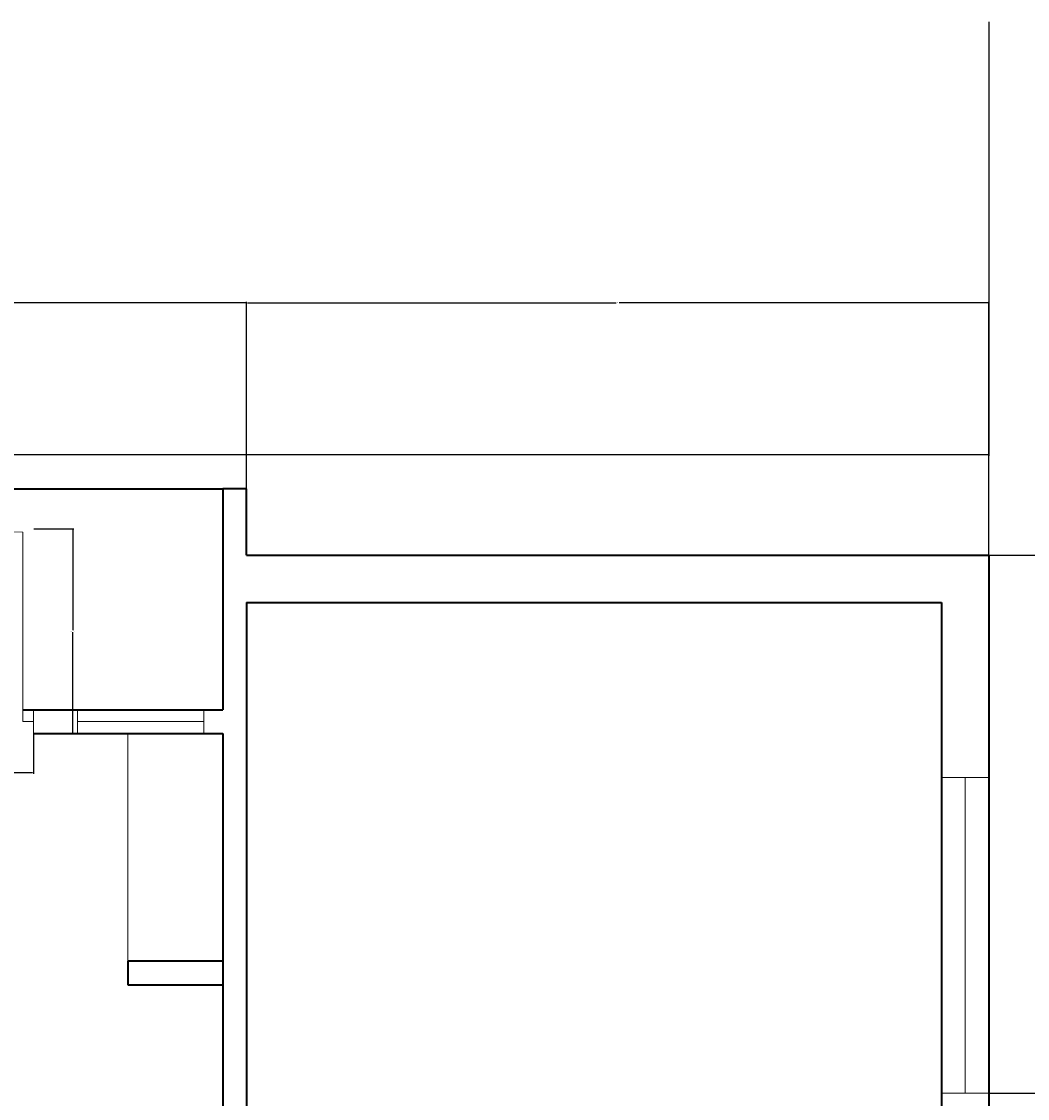
# Model space of a CAD drawing. Units: inches. Extents: x 2250 to 3547, y 1387 to 2604.
# Tile 9 of 11: x 3100 to 3291, y 2129 to 2334. Entities that reach past the tile are written whole.
import ezdxf

# ---------------------------------------------------------------- set-up
doc = ezdxf.new("R2010")
doc.units = ezdxf.units.IN
for name, color, linetype, lineweight in [('A-ANNO-DIMS', 2, 'Continuous', 18), ('A-DOOR', 3, 'Continuous', 18), ('A-FLOR-CASE', 9, 'Continuous', 18), ('A-GLAZ', 4, 'Continuous', 18), ('A-WALL', 7, 'Continuous', 35)]:
    doc.layers.add(name, color=color, linetype=linetype, lineweight=lineweight)
doc.styles.get("Standard").update_dxf_attribs({"font": 'arial.ttf'})
doc.dimstyles.get("Standard").update_dxf_attribs({"dimtxt": 0.18, "dimasz": 0.18, "dimexe": 0.18, "dimexo": 0.0625, "dimgap": 0.09, "dimtad": 0, "dimtih": 1, "dimtoh": 1, "dimdec": 4, "dimzin": 0, "dimdsep": 46, "dimtxsty": 'Standard', "dimcen": 0.09, "dimadec": 0, "dimazin": 0, "dimtfac": 1, "dimtdec": 4, "dimtofl": 0, "dimtmove": 0, "dimatfit": 3, "dimfxl": 1, "dimtolj": 1, "dimtzin": 0, "dimarcsym": 0})

# ---------------------------------------------------------------- blocks, each defined once
blk = doc.blocks.new('WIN-24-SHALLOW')
for p, q in [((0, 4.5), (0, 0)), ((24, 2.25), (24, 4.5)), ((24, 4.5), (24, 0)), ((0, 0), (0, 2.25)), ((0, 2.25), (24, 2.25))]:
    blk.add_line(p, q)
blk = doc.blocks.new('WIN-60-ALT-JAMB')
for p, q in [((9, 60), (0, 60)), ((0, 60), (4.5, 60)), ((4.5, 60), (4.5, 0)), ((4.5, 0), (0, 0)), ((0, 0), (9, 0))]:
    blk.add_line(p, q)
blk = doc.blocks.new('DOOR-ENTRY-DOUBLE-NORTH')
for p, q in [((2, 2.25), (2, 38.25)), ((47.76, 2.25), (47.76, 38.25)), ((0, 4.5), (0, 0)), ((49.76, 4.5), (49.76, 0)), ((0, 0), (0, 2.25)), ((0, 2.25), (2, 2.25)), ((49.76, 2.25), (47.76, 2.25)), ((49.76, 0), (49.76, 2.25))]:
    blk.add_line(p, q)
for centre, radius, start, end in [((2, 13.14), 25.11, 25.0388, 90), ((46.3, 15.04), 23.26, 86.4027, 157.9547)]:
    blk.add_arc(centre, radius, start, end)
blk = doc.blocks.new('*D40')
at = {"layer": 'A-ANNO-DIMS', "color": 0, "lineweight": -2, "transparency": 16777216}
for p, q in [((3052.42, 2198.61), (3052.42, 2191.03)), ((3102.18, 2198.61), (3102.18, 2191.03)), ((3052.6, 2191.21), (3076.31, 2191.21)), ((3102, 2191.21), (3078.28, 2191.21))]:
    blk.add_line(p, q, dxfattribs=at)
at = {"layer": 'A-ANNO-DIMS', "color": 0, "transparency": 16777216}
for points in [[(3052.6, 2191.24), (3052.6, 2191.18), (3052.42, 2191.21)], [(3102, 2191.24), (3102, 2191.18), (3102.18, 2191.21)]]:
    blk.add_solid(points, dxfattribs=at)
at = {"layer": 'Defpoints', "color": 0, "transparency": 16777216}
for p in [(3052.42, 2198.68), (3102.18, 2198.68), (3102.18, 2191.21)]:
    blk.add_point(p, dxfattribs=at)
at = {"layer": 'A-ANNO-DIMS', "color": 0, "transparency": 16777216, "insert": (3077.3, 2191.21), "char_height": 0.18, "attachment_point": 5}
blk.add_mtext('\\A1;ENTRY 50 TYP.', dxfattribs=at)
blk = doc.blocks.new('*D41')
at = {"layer": 'A-ANNO-DIMS', "color": 0, "lineweight": -2, "transparency": 16777216}
for p, q in [((3102.24, 2237.55), (3109.82, 2237.55)), ((3109.64, 2237.37), (3109.64, 2218.3)), ((3109.64, 2198.86), (3109.64, 2217.93)), ((3102.24, 2198.68), (3109.82, 2198.68))]:
    blk.add_line(p, q, dxfattribs=at)
at = {"layer": 'A-ANNO-DIMS', "color": 0, "transparency": 16777216}
for points in [[(3109.61, 2237.37), (3109.67, 2237.37), (3109.64, 2237.55)], [(3109.61, 2198.86), (3109.67, 2198.86), (3109.64, 2198.68)]]:
    blk.add_solid(points, dxfattribs=at)
at = {"layer": 'Defpoints', "color": 0, "transparency": 16777216}
for p in [(3102.18, 2237.55), (3109.64, 2237.55), (3102.18, 2198.68)]:
    blk.add_point(p, dxfattribs=at)
at = {"layer": 'A-ANNO-DIMS', "color": 0, "transparency": 16777216, "insert": (3109.64, 2218.12), "char_height": 0.18, "attachment_point": 5}
blk.add_mtext('\\A1;39 TYP.', dxfattribs=at)
blk = doc.blocks.new('*D90')
at = {"layer": 'A-ANNO-DIMS', "color": 0, "lineweight": -2, "transparency": 16777216}
for p, q in [((3283.69, 2130.34), (3370.22, 2130.34)), ((3370.04, 2130.16), (3370.04, 2093.38)), ((3370.04, 2056.23), (3370.04, 2093.01)), ((3283.69, 2056.05), (3370.22, 2056.05))]:
    blk.add_line(p, q, dxfattribs=at)
at = {"layer": 'A-ANNO-DIMS', "color": 0, "transparency": 16777216}
for points in [[(3370.01, 2130.16), (3370.07, 2130.16), (3370.04, 2130.34)], [(3370.01, 2056.23), (3370.07, 2056.23), (3370.04, 2056.05)]]:
    blk.add_solid(points, dxfattribs=at)
at = {"layer": 'Defpoints', "color": 0, "transparency": 16777216}
for p in [(3283.63, 2130.34), (3370.04, 2130.34), (3283.63, 2056.05)]:
    blk.add_point(p, dxfattribs=at)
at = {"layer": 'A-ANNO-DIMS', "color": 0, "transparency": 16777216, "insert": (3370.04, 2093.2), "char_height": 0.18, "attachment_point": 5}
blk.add_mtext('\\A1;74.29', dxfattribs=at)
blk = doc.blocks.new('*D91')
at = {"layer": 'A-ANNO-DIMS', "color": 0, "lineweight": -2, "transparency": 16777216}
for p, q in [((3283.69, 2232.56), (3370.22, 2232.56)), ((3370.04, 2232.38), (3370.04, 2181.63)), ((3370.04, 2130.52), (3370.04, 2181.27)), ((3283.69, 2130.34), (3370.22, 2130.34))]:
    blk.add_line(p, q, dxfattribs=at)
at = {"layer": 'A-ANNO-DIMS', "color": 0, "transparency": 16777216}
for points in [[(3370.01, 2232.38), (3370.07, 2232.38), (3370.04, 2232.56)], [(3370.01, 2130.52), (3370.07, 2130.52), (3370.04, 2130.34)]]:
    blk.add_solid(points, dxfattribs=at)
at = {"layer": 'Defpoints', "color": 0, "transparency": 16777216}
for p in [(3283.63, 2232.56), (3370.04, 2232.56), (3283.63, 2130.34)]:
    blk.add_point(p, dxfattribs=at)
at = {"layer": 'A-ANNO-DIMS', "color": 0, "transparency": 16777216, "insert": (3370.04, 2181.45), "char_height": 0.18, "attachment_point": 5}
blk.add_mtext('\\A1;102.22', dxfattribs=at)
blk = doc.blocks.new('*D93')
at = {"layer": 'A-ANNO-DIMS', "color": 0, "lineweight": -2, "transparency": 16777216}
for p, q in [((3001.63, 2245.24), (3001.63, 2280.71)), ((3001.81, 2280.53), (3071.87, 2280.53)), ((3142.45, 2280.53), (3072.39, 2280.53)), ((3142.63, 2245.24), (3142.63, 2280.71))]:
    blk.add_line(p, q, dxfattribs=at)
at = {"layer": 'A-ANNO-DIMS', "color": 0, "transparency": 16777216}
for points in [[(3001.81, 2280.56), (3001.81, 2280.5), (3001.63, 2280.53)], [(3142.45, 2280.56), (3142.45, 2280.5), (3142.63, 2280.53)]]:
    blk.add_solid(points, dxfattribs=at)
at = {"layer": 'Defpoints', "color": 0, "transparency": 16777216}
for p in [(3142.63, 2280.53), (3001.63, 2245.18), (3142.63, 2245.18)]:
    blk.add_point(p, dxfattribs=at)
at = {"layer": 'A-ANNO-DIMS', "color": 0, "transparency": 16777216, "insert": (3072.13, 2280.53), "char_height": 0.18, "attachment_point": 5}
blk.add_mtext('\\A1;141', dxfattribs=at)
blk = doc.blocks.new('*D94')
at = {"layer": 'A-ANNO-DIMS', "color": 0, "lineweight": -2, "transparency": 16777216}
for p, q in [((3142.63, 2245.24), (3142.63, 2280.71)), ((3142.81, 2280.53), (3212.87, 2280.53)), ((3283.45, 2280.53), (3213.39, 2280.53)), ((3283.63, 2232.63), (3283.63, 2280.71))]:
    blk.add_line(p, q, dxfattribs=at)
at = {"layer": 'A-ANNO-DIMS', "color": 0, "transparency": 16777216}
for points in [[(3142.81, 2280.56), (3142.81, 2280.5), (3142.63, 2280.53)], [(3283.45, 2280.56), (3283.45, 2280.5), (3283.63, 2280.53)]]:
    blk.add_solid(points, dxfattribs=at)
at = {"layer": 'Defpoints', "color": 0, "transparency": 16777216}
for p in [(3283.63, 2280.53), (3142.63, 2245.18), (3283.63, 2232.56)]:
    blk.add_point(p, dxfattribs=at)
at = {"layer": 'A-ANNO-DIMS', "color": 0, "transparency": 16777216, "insert": (3213.13, 2280.53), "char_height": 0.18, "attachment_point": 5}
blk.add_mtext('\\A1;141', dxfattribs=at)
blk = doc.blocks.new('*D108')
at = {"layer": 'A-ANNO-DIMS', "color": 0, "lineweight": -2, "transparency": 16777216}
for p, q in [((2851.63, 2333.89), (2851.63, 2251.45)), ((3283.63, 2333.89), (3283.63, 2251.45)), ((2851.81, 2251.63), (3067.34, 2251.63)), ((3283.45, 2251.63), (3067.92, 2251.63))]:
    blk.add_line(p, q, dxfattribs=at)
at = {"layer": 'A-ANNO-DIMS', "color": 0, "transparency": 16777216}
for points in [[(2851.81, 2251.66), (2851.81, 2251.6), (2851.63, 2251.63)], [(3283.45, 2251.66), (3283.45, 2251.6), (3283.63, 2251.63)]]:
    blk.add_solid(points, dxfattribs=at)
at = {"layer": 'Defpoints', "color": 0, "transparency": 16777216}
for p in [(2851.63, 2333.95), (3283.63, 2333.95), (3283.63, 2251.63)]:
    blk.add_point(p, dxfattribs=at)
at = {"layer": 'A-ANNO-DIMS', "color": 0, "transparency": 16777216, "insert": (3067.63, 2251.63), "char_height": 0.18, "attachment_point": 5}
blk.add_mtext('\\A1;432', dxfattribs=at)

msp = doc.modelspace()

# ---------------------------------------------------------------- linework, layer by layer
at = {"layer": 'A-FLOR-CASE'}
msp.add_line((3120.1237, 2155.4117), (3120.1237, 2198.6762), dxfattribs=at)
at = {"layer": 'A-WALL'}
for p, q in [((3006.1288, 2245.1762), (3138.1288, 2245.1762)), ((3138.1288, 2245.1762), (3138.1288, 2203.1762)), ((3142.6288, 2245.1762), (3138.1288, 2245.1762)), ((3138.1288, 2245.1762), (3138.1288, 2232.5639)), ((3142.6288, 2232.5639), (3142.6288, 2245.1762)), ((3142.6288, 2232.5639), (3283.6288, 2232.5639)), ((3283.6288, 2232.5639), (3283.6288, 1543.9245)), ((3142.6288, 2223.5639), (3142.6288, 2094.5639)), ((3142.6288, 2223.5639), (3274.6288, 2223.5639)), ((3274.6288, 2223.5639), (3274.6288, 2094.5639)), ((3100.1799, 2203.1762), (3138.1288, 2203.1762)), ((3102.1799, 2198.6762), (3138.1288, 2198.6762)), ((3138.1288, 2198.6762), (3138.1288, 2090.0639)), ((3138.1288, 2155.4117), (3120.1237, 2155.4117)), ((3120.1237, 2155.4117), (3120.1237, 2150.9117)), ((3120.1237, 2150.9117), (3138.1288, 2150.9117))]:
    msp.add_line(p, q, dxfattribs=at)

# ---------------------------------------------------------------- block references
at = {"layer": 'A-DOOR'}
msp.add_blockref('DOOR-ENTRY-DOUBLE-NORTH', (3052.4171, 2198.6762), dxfattribs=at)
at = {"layer": 'A-GLAZ'}
for name, p in [('WIN-24-SHALLOW', (3110.5545, 2198.6762)), ('WIN-60-ALT-JAMB', (3274.6288, 2130.3411))]:
    msp.add_blockref(name, p, dxfattribs=at)

# ---------------------------------------------------------------- dimensions: what is measured, and where the dimension line sits
at = {"layer": 'A-ANNO-DIMS'}
for base, p1, p2, picture, middle in [((3283.6288, 2251.631), (2851.6288, 2333.9493), (3283.6288, 2333.9493), '*D108', (3067.6288, 2251.631)), ((3142.6288, 2280.5262), (3001.6288, 2245.1762), (3142.6288, 2245.1762), '*D93', (3072.1288, 2280.5262)), ((3283.6288, 2280.5262), (3142.6288, 2245.1762), (3283.6288, 2232.5639), '*D94', (3213.1288, 2280.5262))]:
    dim = msp.add_linear_dim(base=base, p1=p1, p2=p2, dimstyle='Standard', override={"dimdec": 0, "dimlfac": 1, "dimrnd": 0, "dimzin": 0, "dimdsep": 46, "dimlunit": 2}, dxfattribs=at)
    dim.commit()
    dim.dimension.update_dxf_attribs({"geometry": picture, "text_midpoint": middle})
dim = msp.add_linear_dim(base=(3109.6443, 2237.5541), p1=(3102.1799, 2198.6762), p2=(3102.1799, 2237.5541), angle=90, text='<> TYP.', dimstyle='Standard', override={"dimdec": 0, "dimlfac": 1, "dimrnd": 0, "dimzin": 0, "dimdsep": 46, "dimlunit": 2}, dxfattribs=at)
dim.commit()
dim.dimension.update_dxf_attribs({"geometry": '*D41', "text_midpoint": (3109.6443, 2218.1151)})
for base, p1, p2, picture, middle in [((3370.0441, 2232.5639), (3283.6288, 2130.3411), (3283.6288, 2232.5639), '*D91', (3370.0441, 2181.4525)), ((3370.0441, 2130.3411), (3283.6288, 2056.0503), (3283.6288, 2130.3411), '*D90', (3370.0441, 2093.1957))]:
    dim = msp.add_linear_dim(base=base, p1=p1, p2=p2, angle=90, dimstyle='Standard', override={"dimdec": 2, "dimlfac": 1, "dimrnd": 0, "dimzin": 0, "dimdsep": 46, "dimlunit": 2}, dxfattribs=at)
    dim.commit()
    dim.dimension.update_dxf_attribs({"geometry": picture, "text_midpoint": middle})
dim = msp.add_linear_dim(base=(3102.1799, 2191.2118), p1=(3052.4171, 2198.6762), p2=(3102.1799, 2198.6762), text='ENTRY <> TYP.', dimstyle='Standard', override={"dimdec": 0, "dimlfac": 1, "dimrnd": 0, "dimzin": 0, "dimdsep": 46, "dimlunit": 2}, dxfattribs=at)
dim.commit()
dim.dimension.update_dxf_attribs({"geometry": '*D40', "text_midpoint": (3077.2985, 2191.2118)})

doc.saveas('drawing.dxf')
